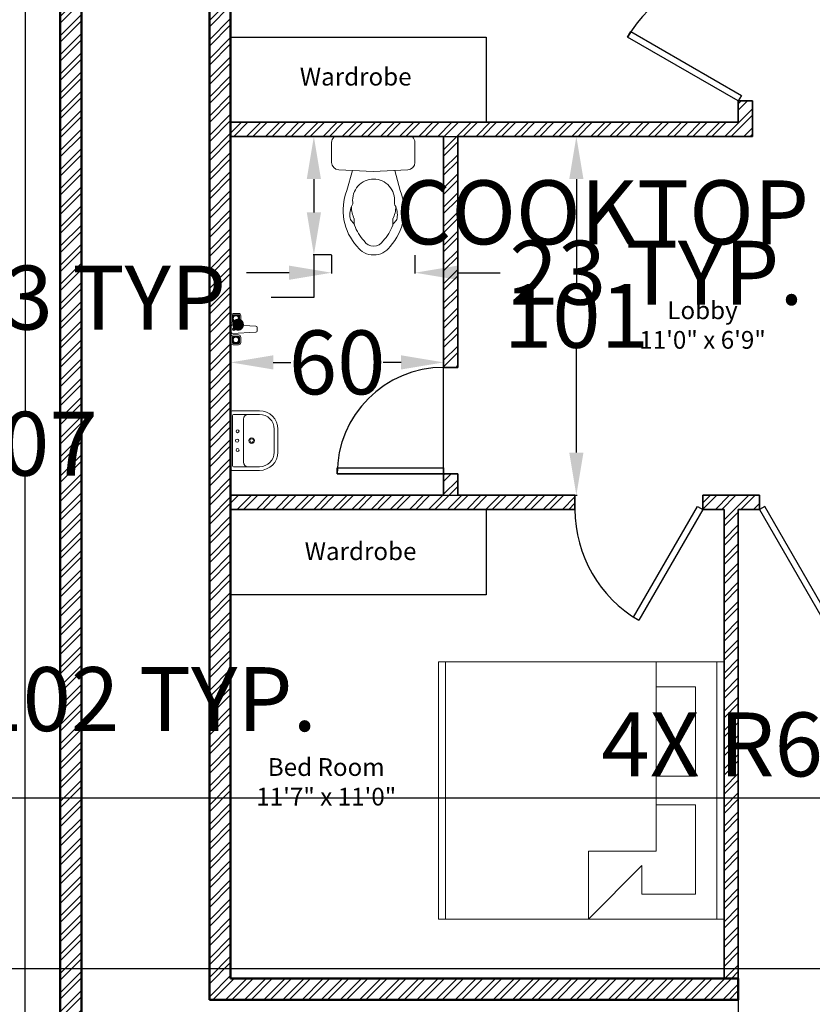
# Model space of a CAD drawing. Units: inches. Extents: x 73 to 1216, y -495 to 328.
# Tile 5 of 9: x 569 to 792, y -232 to 45. Entities that reach past the tile are written whole.
import ezdxf

# ---------------------------------------------------------------- set-up
doc = ezdxf.new("R2010")
doc.units = ezdxf.units.IN
for name, color, linetype, lineweight in [('A-ANNO-DIMS', 2, 'Continuous', 18), ('A-AREA-IDEN', 7, 'Continuous', 18), ('A-DOOR', 3, 'Continuous', 25), ('A-FLOR-CASE', 2, 'Continuous', 25), ('A-FLOR-EDGE', 7, 'Continuous', 25), ('A-FLOR-FIXT', 9, 'Continuous', 18), ('A-WALL-PATT', 8, 'Continuous', 13), ('Furniture', 2, 'Continuous', 18), ('Inner Walls', 5, 'Continuous', 35), ('Outer Walls', 1, 'Continuous', 50), ('Text-T18', 7, 'Continuous', 18)]:
    doc.layers.add(name, color=color, linetype=linetype, lineweight=lineweight)
doc.styles.get("Standard").update_dxf_attribs({"font": 'arial.ttf'})
doc.dimstyles.get("Standard").update_dxf_attribs({"dimtxt": 18, "dimasz": 12, "dimexe": 0.18, "dimexo": 0.0625, "dimgap": 0.09, "dimtad": 0, "dimtih": 1, "dimtoh": 1, "dimdec": 0, "dimzin": 0, "dimdsep": 46, "dimlunit": 3, "dimtxsty": 'Standard', "dimcen": 0.09, "dimadec": 0, "dimazin": 0, "dimtfac": 1, "dimtdec": 0, "dimtofl": 0, "dimtmove": 0, "dimatfit": 3, "dimfxl": 1, "dimtolj": 1, "dimtzin": 0, "dimarcsym": 0})
pattern_1 = [(45, (-647.324, -1257.0093), (-2.694077, 2.694077), []), (45, (-645.528, -1257.0093), (-2.694077, 2.694077), [])]

# ---------------------------------------------------------------- blocks, each defined once
blk = doc.blocks.new('*U2')
for p, q in [((0, 0), (0, -4)), ((36, 0), (36, -4))]:
    blk.add_line(p, q)
blk.add_lwpolyline([(0, 0), (18, 31.18), (19.52, 30.3), (1.52, -0.88)], close=True)
blk.add_arc((0, 0), 36, 0, 60)
blk = doc.blocks.new('*U22')
for p, q in [((0, 0), (0, -4)), ((30, 0), (30, -4))]:
    blk.add_line(p, q)
blk.add_lwpolyline([(0, 0), (0, 30), (1.75, 30), (1.75, 0)], close=True)
blk.add_arc((0, 0), 30, 0, 90)
blk = doc.blocks.new('*U4')
for p, q in [((0, 0), (0, -4)), ((40, 0), (40, -4))]:
    blk.add_line(p, q)
blk.add_lwpolyline([(0, 0), (20, 34.64), (21.52, 33.77), (1.52, -0.88)], close=True)
blk.add_arc((0, 0), 40, 0, 60)
blk = doc.blocks.new('A$C1308471B')
at = {"ltscale": 20}
for p, q in [((0, 0.4607), (0, 0.0186)), ((0.0354, 0.4793), (0.1495, 0.4793)), ((0.2013, 0.2397), (0.1923, 0.4384)), ((0.1957, 0.3639), (0.3109, 0.3953)), ((0.5021, 0.3528), (0.4724, 0.3528)), ((0.4982, 0.3575), (0.4822, 0.3709)), ((0.2013, 0.2397), (0.1923, 0.0409)), ((0.1959, 0.1193), (0.3109, 0.0879)), ((0.5021, 0.1304), (0.4724, 0.1304)), ((0.4982, 0.1257), (0.4822, 0.1123)), ((0.0354, 0), (0.1495, 0))]:
    blk.add_line(p, q, dxfattribs=at)
for centre, radius, start, end in [((0.006, 0.4607), 0.006, 136.5269, 180), ((0.0354, 0.4328), 0.0465, 90, 136.5269), ((0.1495, 0.4365), 0.0429, 2.5755, 90), ((0.4248, 0.1104), 0.3068, 47.4135, 111.7924), ((0.3654, 0.2416), 0.1206, 83.3523, 180), ((0.3823, 0.3868), 0.0255, 263.3523, 298.5742), ((0.4494, 0.2636), 0.1148, 79.3968, 118.5742), ((0.405, 0.2159), 0.153, 63.502, 90.4522), ((0.4658, 0.3513), 0.0255, 50, 79.3968), ((0.5146, 0.377), 0.0255, 230, 251.3881), ((0.5021, 0.3273), 0.0255, 70.3751, 90), ((0.4248, 0.1104), 0.2558, 46.612, 70.3751), ((0.5654, 0.2416), 0.065, 0, 57.2974), ((0.5654, 0.2416), 0.116, 0, 54.7115), ((0.3654, 0.2416), 0.1206, 180, 276.6477), ((0.5654, 0.2416), 0.065, 302.7026, 0), ((0.5654, 0.2416), 0.116, 305.2885, 0), ((0.4248, 0.3728), 0.2558, 289.6249, 313.388), ((0.4248, 0.3728), 0.3068, 248.2076, 312.5865), ((0.3823, 0.0964), 0.0255, 61.4258, 96.6477), ((0.4494, 0.2196), 0.1148, 241.4258, 280.6032), ((0.405, 0.2673), 0.153, 269.5478, 296.498), ((0.5146, 0.1062), 0.0255, 108.6119, 130), ((0.5021, 0.1559), 0.0255, 270, 289.6249), ((0.4658, 0.1319), 0.0255, 280.6032, 310), ((0.006, 0.0186), 0.006, 180, 223.4731), ((0.0354, 0.0465), 0.0465, 223.4731, 270), ((0.1495, 0.0429), 0.0429, 270, 357.4245)]:
    blk.add_arc(centre, radius, start, end, dxfattribs=at)
blk = doc.blocks.new('A$C57EA129C')
for p, q in [((0, 0.4428), (0, 0.1782)), ((0.016, 0.4589), (0.5631, 0.4589)), ((0.0356, 0.4321), (0.0356, 0.2896)), ((0.0445, 0.441), (0.5346, 0.441)), ((0.5435, 0.4321), (0.5435, 0.2896)), ((0.5791, 0.4428), (0.5791, 0.1782)), ((0.0356, 0.2896), (0.0356, 0.1782)), ((0.0802, 0.3341), (0.499, 0.3341)), ((0.5435, 0.2896), (0.5435, 0.1782)), ((0.1782, 0.0356), (0.4009, 0.0356)), ((0.1782, 0), (0.4009, 0))]:
    blk.add_line(p, q)
for centre, radius in [((0.1982, 0.392), 0.0143), ((0.2896, 0.3965), 0.0156), ((0.3809, 0.392), 0.0143), ((0.2896, 0.2545), 0.0267), ((0.2896, 0.2545), 0.0178)]:
    blk.add_circle(centre, radius)
for centre, radius, start, end in [((0.016, 0.4428), 0.016, 90, 180), ((0.0445, 0.4321), 0.00891, 90, 180), ((0.5346, 0.4321), 0.00891, 0, 90), ((0.5631, 0.4428), 0.016, 0, 90), ((0.0802, 0.2896), 0.0445, 90, 180), ((0.499, 0.2896), 0.0445, 0, 90), ((0.1782, 0.1782), 0.1782, 180, 270), ((0.1782, 0.1782), 0.1426, 180, 270), ((0.4009, 0.1782), 0.1782, 270, 0), ((0.4009, 0.1782), 0.1426, 270, 0)]:
    blk.add_arc(centre, radius, start, end)
blk = doc.blocks.new('A$C68D75330')
for p, q in [((0.1549, 0.4064), (0.1549, 0.4514)), ((0.1674, 0.4039), (0.1674, 0.4539)), ((0.1724, 0.4589), (0.2224, 0.4589)), ((0.1749, 0.4714), (0.2199, 0.4714)), ((0.2274, 0.4539), (0.2274, 0.4039)), ((0.2399, 0.4514), (0.2399, 0.4064)), ((0.2644, 0.2559), (0.2524, 0.4614)), ((0.2749, 0.4714), (0.3049, 0.4714)), ((0.3274, 0.4614), (0.3155, 0.2559)), ((0.3399, 0.4514), (0.3399, 0.4064)), ((0.3524, 0.4539), (0.3524, 0.4039)), ((0.4074, 0.4589), (0.3574, 0.4589)), ((0.4049, 0.4714), (0.3599, 0.4714)), ((0.4124, 0.4039), (0.4124, 0.4539)), ((0.4249, 0.4064), (0.4249, 0.4514)), ((0.2224, 0.3989), (0.1724, 0.3989)), ((0.2199, 0.3864), (0.1749, 0.3864)), ((0.3574, 0.3989), (0.4074, 0.3989)), ((0.3599, 0.3864), (0.4049, 0.3864)), ((0.3055, 0.2464), (0.2744, 0.2464))]:
    blk.add_line(p, q)
for centre, radius in [((0.1974, 0.4289), 0.03), ((0.1974, 0.4289), 0.0232), ((0.2899, 0.4464), 0.0125), ((0.2899, 0.4464), 0.00625), ((0.3824, 0.4289), 0.03), ((0.3824, 0.4289), 0.0232)]:
    blk.add_circle(centre, radius)
for centre, radius, start, end in [((0.1749, 0.4514), 0.02, 90, 180), ((0.1724, 0.4539), 0.005, 90, 180), ((0.2199, 0.4514), 0.02, 0, 90), ((0.2224, 0.4539), 0.005, 0, 90), ((0.2736, 0.4441), 0.0273, 87.19754, 140.72744), ((0.3063, 0.4441), 0.0273, 39.27256, 92.80246), ((0.3599, 0.4514), 0.02, 90, 180), ((0.3574, 0.4539), 0.005, 90, 180), ((0.4049, 0.4514), 0.02, 0, 90), ((0.4074, 0.4539), 0.005, 0, 90), ((0.1749, 0.4064), 0.02, 180, 270), ((0.1724, 0.4039), 0.005, 180, 270), ((0.2199, 0.4064), 0.02, 270, 0), ((0.2224, 0.4039), 0.005, 270, 0), ((0.3599, 0.4064), 0.02, 180, 270), ((0.3574, 0.4039), 0.005, 180, 270), ((0.4049, 0.4064), 0.02, 270, 0), ((0.4074, 0.4039), 0.005, 270, 0), ((0.2744, 0.2564), 0.01, 183.3274, 270), ((0.3055, 0.2564), 0.01, 270, 356.6726)]:
    blk.add_arc(centre, radius, start, end)
blk = doc.blocks.new('KING-00')
for p, q in [((-0.8967, -0.947), (-0.8967, 0.8818)), ((0.6019, 0.8818), (0.6019, -0.4644)), ((1.0337, -0.947), (1.0337, 0.8818)), ((0.6019, 0.704), (0.8813, 0.704)), ((0.8813, 0.069), (0.8813, 0.704)), ((0.6019, 0.069), (0.8813, 0.069)), ((0.8813, -0.1342), (0.6019, -0.1342)), ((0.8813, -0.7692), (0.8813, -0.1342)), ((0.1193, -0.4644), (0.1193, -0.947)), ((0.6019, -0.4644), (0.1193, -0.4644)), ((0.1193, -0.947), (0.5003, -0.566)), ((0.5003, -0.7692), (0.5003, -0.566)), ((0.5003, -0.7692), (0.8813, -0.7692))]:
    blk.add_line(p, q)
blk.add_lwpolyline([(-0.9475, -0.947), (-0.9475, 0.8818), (1.0845, 0.8818), (1.0845, -0.947)], close=True)
blk = doc.blocks.new('WARDROBE-72X24')
blk.add_lwpolyline([(0, 24), (72, 24), (72, 0), (0, 0)], close=True)
blk = doc.blocks.new('*D26')
at = {"layer": 'A-ANNO-DIMS', "color": 0, "lineweight": -2, "transparency": 16777216}
for p, q in [((690.69, 91.4), (690.69, 79.21)), ((771.16, 91.4), (771.16, 79.21)), ((702.69, 79.39), (759.16, 79.39)), ((771.16, 79.39), (783.16, 79.39))]:
    blk.add_line(p, q, dxfattribs=at)
at = {"layer": 'A-ANNO-DIMS', "color": 0, "transparency": 16777216}
for points in [[(702.69, 81.39), (702.69, 77.39), (690.69, 79.39)], [(759.16, 81.39), (759.16, 77.39), (771.16, 79.39)]]:
    blk.add_solid(points, dxfattribs=at)
at = {"layer": 'Defpoints', "color": 0, "transparency": 16777216}
for p in [(690.69, 91.46), (771.16, 91.46), (771.16, 79.39)]:
    blk.add_point(p, dxfattribs=at)
at = {"layer": 'A-ANNO-DIMS', "color": 0, "transparency": 16777216, "insert": (890.24, 79.39), "char_height": 18, "attachment_point": 5}
blk.add_mtext('\\A1;KING BED 80 TYP.', dxfattribs=at)
blk = doc.blocks.new('*D28')
at = {"layer": 'A-ANNO-DIMS', "color": 0, "lineweight": -2, "transparency": 16777216}
for p, q in [((520.8, -95.45), (536.15, -95.45)), ((535.97, -107.45), (535.97, -136.81)), ((535.97, -184.97), (535.97, -155.61)), ((520.8, -196.97), (536.15, -196.97))]:
    blk.add_line(p, q, dxfattribs=at)
at = {"layer": 'A-ANNO-DIMS', "color": 0, "transparency": 16777216}
for points in [[(533.97, -107.45), (537.97, -107.45), (535.97, -95.45)], [(533.97, -184.97), (537.97, -184.97), (535.97, -196.97)]]:
    blk.add_solid(points, dxfattribs=at)
at = {"layer": 'Defpoints', "color": 0, "transparency": 16777216}
for p in [(520.74, -95.45), (520.74, -196.97), (535.97, -196.97)]:
    blk.add_point(p, dxfattribs=at)
at = {"layer": 'A-ANNO-DIMS', "color": 0, "transparency": 16777216, "insert": (535.97, -146.21), "char_height": 18, "attachment_point": 5}
blk.add_mtext('\\A1;SECTIONAL 102 TYP.', dxfattribs=at)
blk = doc.blocks.new('*D30')
at = {"layer": 'A-ANNO-DIMS', "color": 0, "lineweight": -2, "transparency": 16777216}
for p, q in [((656.55, 12.18), (651.43, 12.18)), ((651.61, 0.18), (651.61, -9.18)), ((656.55, -21.18), (651.43, -21.18)), ((651.61, -21.18), (651.61, -33.18)), ((651.61, -33.18), (639.61, -33.18))]:
    blk.add_line(p, q, dxfattribs=at)
at = {"layer": 'A-ANNO-DIMS', "color": 0, "transparency": 16777216}
for points in [[(649.61, 0.18), (653.61, 0.18), (651.61, 12.18)], [(649.61, -9.18), (653.61, -9.18), (651.61, -21.18)]]:
    blk.add_solid(points, dxfattribs=at)
at = {"layer": 'Defpoints', "color": 0, "transparency": 16777216}
for p in [(656.61, 12.18), (651.61, -21.18), (656.61, -21.18)]:
    blk.add_point(p, dxfattribs=at)
at = {"layer": 'A-ANNO-DIMS', "color": 0, "transparency": 16777216, "insert": (570.9, -33.18), "char_height": 18, "attachment_point": 5}
blk.add_mtext('\\A1;WC 33 TYP.', dxfattribs=at)
blk = doc.blocks.new('*D31')
at = {"layer": 'A-ANNO-DIMS', "color": 0, "lineweight": -2, "transparency": 16777216}
for p, q in [((656.61, -21.24), (656.61, -26.36)), ((680.08, -21.24), (680.08, -26.36)), ((644.61, -26.18), (632.61, -26.18)), ((692.08, -26.18), (704.08, -26.18))]:
    blk.add_line(p, q, dxfattribs=at)
at = {"layer": 'A-ANNO-DIMS', "color": 0, "transparency": 16777216}
for points in [[(644.61, -24.18), (644.61, -28.18), (656.61, -26.18)], [(692.08, -24.18), (692.08, -28.18), (680.08, -26.18)]]:
    blk.add_solid(points, dxfattribs=at)
at = {"layer": 'Defpoints', "color": 0, "transparency": 16777216}
for p in [(656.61, -21.18), (680.08, -21.18), (680.08, -26.18)]:
    blk.add_point(p, dxfattribs=at)
at = {"layer": 'A-ANNO-DIMS', "color": 0, "transparency": 16777216, "insert": (748.13, -26.18), "char_height": 18, "attachment_point": 5}
blk.add_mtext('\\A1;23 TYP.', dxfattribs=at)
blk = doc.blocks.new('*D42')
at = {"layer": 'A-ANNO-DIMS', "color": 0, "lineweight": -2, "transparency": 16777216}
for p, q in [((903.29, 30.3), (899.05, 30.3)), ((899.23, 18.3), (899.23, 14.82)), ((903.29, 2.82), (899.05, 2.82)), ((899.23, 2.82), (899.23, -9.18)), ((899.23, -9.18), (887.23, -9.18))]:
    blk.add_line(p, q, dxfattribs=at)
at = {"layer": 'A-ANNO-DIMS', "color": 0, "transparency": 16777216}
for points in [[(897.23, 18.3), (901.23, 18.3), (899.23, 30.3)], [(897.23, 14.82), (901.23, 14.82), (899.23, 2.82)]]:
    blk.add_solid(points, dxfattribs=at)
at = {"layer": 'Defpoints', "color": 0, "transparency": 16777216}
for p in [(903.36, 30.3), (899.23, 2.82), (903.36, 2.82)]:
    blk.add_point(p, dxfattribs=at)
at = {"layer": 'A-ANNO-DIMS', "color": 0, "transparency": 16777216, "insert": (777.07, -9.18), "char_height": 18, "attachment_point": 5}
blk.add_mtext('\\A1;COOKTOP 27 TYP.', dxfattribs=at)
blk = doc.blocks.new('*D51')
at = {"layer": 'A-ANNO-DIMS', "color": 0, "lineweight": -2, "transparency": 16777216}
for p, q in [((532.94, 279.18), (570.45, 279.18)), ((570.27, 267.18), (570.27, -65.04)), ((570.27, -415.82), (570.27, -83.6)), ((532.94, -427.82), (570.45, -427.82))]:
    blk.add_line(p, q, dxfattribs=at)
at = {"layer": 'A-ANNO-DIMS', "color": 0, "transparency": 16777216}
for points in [[(568.27, 267.18), (572.27, 267.18), (570.27, 279.18)], [(568.27, -415.82), (572.27, -415.82), (570.27, -427.82)]]:
    blk.add_solid(points, dxfattribs=at)
at = {"layer": 'Defpoints', "color": 0, "transparency": 16777216}
for p in [(532.87, 279.18), (570.27, 279.18), (532.87, -427.82)]:
    blk.add_point(p, dxfattribs=at)
at = {"layer": 'A-ANNO-DIMS', "color": 0, "transparency": 16777216, "insert": (570.27, -74.32), "char_height": 18, "attachment_point": 5}
blk.add_mtext('\\A1;707', dxfattribs=at)
blk = doc.blocks.new('*D53')
at = {"layer": 'A-ANNO-DIMS', "color": 0, "lineweight": -2, "transparency": 16777216}
for p, q in [((580.1, 279.18), (542.58, 279.18)), ((542.76, 267.18), (542.76, -65.04)), ((542.76, -415.82), (542.76, -83.6)), ((580.1, -427.82), (542.58, -427.82))]:
    blk.add_line(p, q, dxfattribs=at)
at = {"layer": 'A-ANNO-DIMS', "color": 0, "transparency": 16777216}
for points in [[(540.76, 267.18), (544.76, 267.18), (542.76, 279.18)], [(540.76, -415.82), (544.76, -415.82), (542.76, -427.82)]]:
    blk.add_solid(points, dxfattribs=at)
at = {"layer": 'Defpoints', "color": 0, "transparency": 16777216}
for p in [(542.76, 279.18), (580.16, 279.18), (580.16, -427.82)]:
    blk.add_point(p, dxfattribs=at)
at = {"layer": 'A-ANNO-DIMS', "color": 0, "transparency": 16777216, "insert": (542.76, -74.32), "char_height": 18, "attachment_point": 5}
blk.add_mtext('\\A1;707', dxfattribs=at)
blk = doc.blocks.new('*D59')
at = {"layer": 'A-ANNO-DIMS', "color": 0, "lineweight": -2, "transparency": 16777216}
for p, q in [((628.16, -88.76), (628.16, -51.24)), ((640.16, -51.42), (645.16, -51.42)), ((676.16, -51.42), (671.17, -51.42)), ((688.16, -88.76), (688.16, -51.24))]:
    blk.add_line(p, q, dxfattribs=at)
at = {"layer": 'A-ANNO-DIMS', "color": 0, "transparency": 16777216}
for points in [[(640.16, -49.42), (640.16, -53.42), (628.16, -51.42)], [(676.16, -49.42), (676.16, -53.42), (688.16, -51.42)]]:
    blk.add_solid(points, dxfattribs=at)
at = {"layer": 'Defpoints', "color": 0, "transparency": 16777216}
for p in [(688.16, -51.42), (628.16, -88.82), (688.16, -88.82)]:
    blk.add_point(p, dxfattribs=at)
at = {"layer": 'A-ANNO-DIMS', "color": 0, "transparency": 16777216, "insert": (658.16, -51.42), "char_height": 18, "attachment_point": 5}
blk.add_mtext('\\A1;60', dxfattribs=at)
blk = doc.blocks.new('*D60')
at = {"layer": 'A-ANNO-DIMS', "color": 0, "lineweight": -2, "transparency": 16777216}
for p, q in [((688.23, 12.18), (725.74, 12.18)), ((725.56, 0.18), (725.56, -29.04)), ((725.56, -76.82), (725.56, -47.6)), ((688.23, -88.82), (725.74, -88.82))]:
    blk.add_line(p, q, dxfattribs=at)
at = {"layer": 'A-ANNO-DIMS', "color": 0, "transparency": 16777216}
for points in [[(723.56, 0.18), (727.56, 0.18), (725.56, 12.18)], [(723.56, -76.82), (727.56, -76.82), (725.56, -88.82)]]:
    blk.add_solid(points, dxfattribs=at)
at = {"layer": 'Defpoints', "color": 0, "transparency": 16777216}
for p in [(688.16, 12.18), (688.16, -88.82), (725.56, -88.82)]:
    blk.add_point(p, dxfattribs=at)
at = {"layer": 'A-ANNO-DIMS', "color": 0, "transparency": 16777216, "insert": (725.56, -38.32), "char_height": 18, "attachment_point": 5}
blk.add_mtext('\\A1;101', dxfattribs=at)
blk = doc.blocks.new('*D67')
at = {"layer": 'A-ANNO-DIMS', "color": 0, "lineweight": -2, "transparency": 16777216}
for p, q in [((798.02113, 227.113801), (798.02113, -465.403699)), ((834.02113, 227.113801), (834.02113, -465.403699)), ((786.02113, -465.223699), (774.02113, -465.223699)), ((846.02113, -465.223699), (858.02113, -465.223699))]:
    blk.add_line(p, q, dxfattribs=at)
at = {"layer": 'A-ANNO-DIMS', "color": 0, "transparency": 16777216}
for points in [[(786.02113, -463.223699), (786.02113, -467.223699), (798.02113, -465.223699)], [(846.02113, -463.223699), (846.02113, -467.223699), (834.02113, -465.223699)]]:
    blk.add_solid(points, dxfattribs=at)
at = {"layer": 'Defpoints', "color": 0, "transparency": 16777216}
for p in [(798.02113, 227.176301), (834.02113, 227.176301), (834.02113, -465.223699)]:
    blk.add_point(p, dxfattribs=at)
at = {"layer": 'A-ANNO-DIMS', "color": 0, "transparency": 16777216, "insert": (816.02113, -465.223699), "char_height": 18, "attachment_point": 5}
blk.add_mtext('\\A1;36', dxfattribs=at)
blk = doc.blocks.new('*D78')
at = {"layer": 'A-ANNO-DIMS', "color": 0, "lineweight": -2, "transparency": 16777216}
for p, q in [((831.3, -174.14), (542.58, -174.14)), ((542.76, -186.14), (542.76, -188.86)), ((542.76, -210.14), (542.76, -207.42)), ((831.3, -222.14), (542.58, -222.14))]:
    blk.add_line(p, q, dxfattribs=at)
at = {"layer": 'A-ANNO-DIMS', "color": 0, "transparency": 16777216}
for points in [[(540.76, -186.14), (544.76, -186.14), (542.76, -174.14)], [(540.76, -210.14), (544.76, -210.14), (542.76, -222.14)]]:
    blk.add_solid(points, dxfattribs=at)
at = {"layer": 'Defpoints', "color": 0, "transparency": 16777216}
for p in [(542.76, -174.14), (831.36, -174.14), (831.36, -222.14)]:
    blk.add_point(p, dxfattribs=at)
at = {"layer": 'A-ANNO-DIMS', "color": 0, "transparency": 16777216, "insert": (542.76, -198.14), "char_height": 18, "attachment_point": 5}
blk.add_mtext('\\A1;48', dxfattribs=at)
blk = doc.blocks.new('*D79')
at = {"layer": 'A-ANNO-DIMS', "color": 0, "lineweight": -2, "transparency": 16777216}
for p, q in [((798.1, -158.97), (810.1, -158.97)), ((810.1, -158.97), (818.61, -167.44)), ((831.27, -180.14), (831.45, -180.14)), ((831.36, -180.23), (831.36, -180.05))]:
    blk.add_line(p, q, dxfattribs=at)
at = {"layer": 'A-ANNO-DIMS', "color": 0, "transparency": 16777216}
blk.add_solid([(820.02, -166.02), (817.19, -168.86), (827.11, -175.91)], dxfattribs=at)
at = {"layer": 'Defpoints', "color": 0, "transparency": 16777216}
for p in [(827.11, -175.91), (831.36, -180.14)]:
    blk.add_point(p, dxfattribs=at)
at = {"layer": 'A-ANNO-DIMS', "color": 0, "transparency": 16777216, "insert": (763.81, -158.97), "char_height": 18, "attachment_point": 5}
blk.add_mtext('\\A1;4X R6', dxfattribs=at)

msp = doc.modelspace()

# ---------------------------------------------------------------- hatches: boundary and pattern name
at = {"layer": 'A-WALL-PATT'}
h = msp.add_hatch(dxfattribs=at)
h.set_pattern_fill('ANSI32', color=256, scale=0.4)
h.set_pattern_definition(pattern_1)
h.paths.add_polyline_path([(586.1647, 273.1763), (924.1647, 273.1763), (924.1647, -421.8237), (753.1647, -421.8237), (753.1647, -427.8237), (930.1647, -427.8237), (930.1647, 279.1763), (580.1647, 279.1763), (580.1647, -427.8237), (633.1647, -427.8237), (633.1647, -421.8237), (586.1647, -421.8237)])
h = msp.add_hatch(dxfattribs=at)
h.set_pattern_fill('ANSI32', color=256, scale=0.4)
h.set_pattern_definition(pattern_1)
h.paths.add_polyline_path([(685.1647, 201.1763), (679.1647, 201.1763), (679.1647, 206.1763), (675.1647, 206.1763), (675.1647, 201.1763), (586.1647, 201.1763), (586.1647, 197.1763), (685.1647, 197.1763)])
h.paths.add_polyline_path([(679.1647, 273.1763), (675.1647, 273.1763), (675.1647, 236.1763), (679.1647, 236.1763)])
h.paths.add_polyline_path([(775.1647, 201.1763), (772.1647, 201.1763), (772.1647, 273.1763), (768.1647, 273.1763), (768.1647, 249.1763), (768.1647, 201.1763), (721.1647, 201.1763), (721.1647, 197.1763), (771.1647, 197.1763), (771.1647, 58.1763), (775.1647, 58.1763)])
h.paths.add_polyline_path([(798.0211, 233.1763), (772.1647, 233.1763), (772.1647, 227.1763), (798.0211, 227.1763)])
h.paths.add_polyline_path([(870.8232, 233.1763), (834.0211, 233.1763), (834.0211, 227.1763), (870.8232, 227.1763)])
h.paths.add_polyline_path([(924.1647, 233.1763), (906.8232, 233.1763), (906.8232, 227.1763), (924.1647, 227.1763)])
h.paths.add_polyline_path([(924.1647, 83.1763), (775.1647, 83.1763), (775.1647, 79.1763), (924.1647, 79.1763)])
h.paths.add_polyline_path([(775.1647, 22.1763), (771.1647, 22.1763), (771.1647, 16.1763), (628.1647, 16.1763), (628.1647, 12.1763), (775.1647, 12.1763)])
h.paths.add_polyline_path([(692.1647, 12.1763), (688.1647, 12.1763), (688.1647, -52.8237), (692.1647, -52.8237)])
h.paths.add_polyline_path([(924.1647, 39.1763), (824.1647, 39.1763), (824.1647, 35.1763), (924.1647, 35.1763)])
h.paths.add_polyline_path([(874.6647, -29.8237), (864.1647, -29.8237), (824.1647, -29.8237), (824.1647, -87.8237), (817.1647, -87.8237), (817.1647, -91.8237), (844.6647, -91.8237), (844.6647, -87.8237), (828.1647, -87.8237), (828.1647, -33.8237), (874.6647, -33.8237)])
h.paths.add_polyline_path([(924.1647, -29.8237), (910.6647, -29.8237), (910.6647, -33.8237), (924.1647, -33.8237)])
h.paths.add_polyline_path([(924.1647, -87.8237), (904.6647, -87.8237), (904.6647, -91.8237), (924.1647, -91.8237)])
h.paths.add_polyline_path([(777.1647, -88.8237), (761.1647, -88.8237), (761.1647, -92.8237), (767.1647, -92.8237), (767.1647, -224.8237), (771.1647, -224.8237), (771.1647, -92.8237), (777.1647, -92.8237)])
h.paths.add_polyline_path([(725.1647, -88.8237), (628.1647, -88.8237), (628.1647, -92.8237), (725.1647, -92.8237)])
h.paths.add_polyline_path([(692.1647, -82.8237), (688.1647, -82.8237), (688.1647, -88.8237), (692.1647, -88.8237)])
h.paths.add_polyline_path([(767.1647, -313.8237), (924.1647, -313.8237), (924.1647, -307.8237), (763.1647, -307.8237), (763.1647, -421.8237), (767.1647, -421.8237)])
h = msp.add_hatch(dxfattribs=at)
h.set_pattern_fill('ANSI32', color=256, scale=0.4)
h.set_pattern_definition(pattern_1)
h.paths.add_polyline_path([(628.1647, 197.1763), (622.1647, 197.1763), (622.1647, -230.8237), (771.1647, -230.8237), (771.1647, -224.8237), (628.1647, -224.8237)])

# ---------------------------------------------------------------- linework, layer by layer
at = {"layer": 'A-FLOR-EDGE'}
msp.add_line((771.1647, -229.8237), (771.1647, -307.8237), dxfattribs=at)
at = {"layer": 'Inner Walls'}
for p, q in [((771.1647, 22.1763), (771.1647, 16.1763)), ((775.1647, 22.1763), (771.1647, 22.1763)), ((775.1647, 22.1763), (775.1647, 12.1763)), ((771.1647, 16.1763), (628.1647, 16.1763)), ((688.1647, 12.1763), (628.1647, 12.1763)), ((688.1647, -52.8237), (688.1647, 12.1763)), ((775.1647, 12.1763), (692.1647, 12.1763)), ((692.1647, -52.8237), (692.1647, 12.1763)), ((692.1647, -52.8237), (688.1647, -52.8237)), ((692.1647, -82.8237), (658.1647, -82.8237)), ((688.1647, -88.8237), (688.1647, -81.0737)), ((692.1647, -88.8237), (692.1647, -82.8237)), ((688.1647, -88.8237), (628.1647, -88.8237)), ((725.1647, -88.8237), (692.1647, -88.8237)), ((725.1647, -92.8237), (725.1647, -88.8237)), ((761.1647, -92.8237), (761.1647, -88.8237)), ((761.1647, -88.8237), (777.1647, -88.8237)), ((777.1647, -88.8237), (777.1647, -92.8237)), ((725.1647, -92.8237), (628.1647, -92.8237)), ((767.1647, -92.8237), (761.1647, -92.8237)), ((767.1647, -224.8237), (767.1647, -92.8237)), ((771.1647, -224.8237), (771.1647, -92.8237)), ((771.1647, -92.8237), (777.1647, -92.8237))]:
    msp.add_line(p, q, dxfattribs=at)
at = {"layer": 'Outer Walls'}
for p, q in [((580.1647, -427.8237), (580.1647, 279.1763)), ((586.1647, -421.8237), (586.1647, 273.1763)), ((622.1647, -230.8237), (622.1647, 197.1763)), ((628.1647, -224.8237), (628.1647, 197.1763)), ((771.1647, -224.8237), (628.1647, -224.8237)), ((771.1647, -224.8237), (771.1647, -230.8237)), ((771.1647, -230.8237), (622.1647, -230.8237))]:
    msp.add_line(p, q, dxfattribs=at)

# ---------------------------------------------------------------- block references
at = {"layer": 'A-DOOR'}
for name, p, rotation in [('*U2', (771.1647, 22.1763), 90), ('*U22', (688.1647, -82.8237), 90.00000000000003), ('*U2', (761.1647, -92.8237), 180)]:
    msp.add_blockref(name, p, dxfattribs=dict(at, rotation=rotation))
at = {"layer": 'A-DOOR', "xscale": -1, "rotation": 180}
msp.add_blockref('*U4', (777.1647, -92.8237), dxfattribs=at)
at = {"layer": 'A-FLOR-CASE'}
for p in [(628.1651, 16.176), (628.1651, -116.824)]:
    msp.add_blockref('WARDROBE-72X24', p, dxfattribs=at)
at = {"layer": 'A-FLOR-FIXT'}
for name, p, xscale, yscale, zscale, rotation in [('A$C1308471B', (656.6088, 12.1763), 48.95497407897215, 48.95497407897215, 48.95497407897215, 269.9999999999999), ('A$C68D75330', (643.6487, -51.536), 32.67217261962217, 32.67217261962217, 32.67217261962217, 89.99999999999999), ('A$C57EA129C', (641.4641, -65.051), -28.98333223671166, 28.98333223671166, 28.98333223671166, 90)]:
    msp.add_blockref(name, p, dxfattribs=dict(at, xscale=xscale, yscale=yscale, zscale=zscale, rotation=rotation))
at = {"layer": 'Furniture', "xscale": 39.60249106241186, "yscale": 39.60249106241186, "zscale": 39.60249106241186}
msp.add_blockref('KING-00', (724.2158, -170.639), dxfattribs=at)

# ---------------------------------------------------------------- texts
at = {"layer": 'A-AREA-IDEN', "char_height": 5, "attachment_point": 3}
for s, insert in [('\\pxqc;{\\fTimes New Roman|b0|i0|c0|p18;Lobby\\P11\'0" x 6\'9"}', (785.6525, -34.2468)), ('\\pxqc;{\\fTimes New Roman|b0|i0|c0|p18;Bed Room \\P11\'7" x 11\'0"}', (679.6433, -162.8344))]:
    msp.add_mtext_dynamic_manual_height_columns(s, width=49.101878, gutter_width=12.5, heights=[0], dxfattribs=dict(at, insert=insert))
at = {"layer": 'Text-T18', "char_height": 5, "attachment_point": 3}
for insert in [(687.9442, 31.5208), (689.3169, -102.0799)]:
    msp.add_mtext_dynamic_manual_height_columns('\\pxqc;{\\fTimes New Roman|b0|i0|c0|p18;Wardrobe}', width=49.101878, gutter_width=12.5, heights=[0], dxfattribs=dict(at, insert=insert))

# ---------------------------------------------------------------- dimensions: what is measured, and where the dimension line sits
at = {"layer": 'A-ANNO-DIMS'}
for base, p1, p2, angle, picture, middle in [((542.7647, 279.1763), (580.1647, -427.8237), (580.1647, 279.1763), 90, '*D53', (542.7647, -74.3237)), ((570.2746, 279.1763), (532.8746, -427.8237), (532.8746, 279.1763), 90, '*D51', (570.2746, -74.3237)), ((725.5647, -88.8237), (688.1647, 12.1763), (688.1647, -88.8237), 270, '*D60', (725.5647, -38.3237)), ((688.1647, -51.4237), (628.1647, -88.8237), (688.1647, -88.8237), 0, '*D59', (658.1647, -51.4237)), ((542.7647, -174.1414), (831.3578, -222.1414), (831.3578, -174.1414), 90, '*D78', (542.7647, -198.1414))]:
    dim = msp.add_linear_dim(base=base, p1=p1, p2=p2, angle=angle, dimstyle='Standard', override={"dimdec": 0, "dimlfac": 1, "dimrnd": 0, "dimzin": 0, "dimdsep": 46, "dimlunit": 2}, dxfattribs=at)
    dim.commit()
    dim.dimension.update_dxf_attribs({"geometry": picture, "text_midpoint": middle})
dim = msp.add_linear_dim(base=(834.0211, -465.2237), p1=(798.0211, 227.1763), p2=(834.0211, 227.1763), dimstyle='Standard', override={"dimdec": 0, "dimlfac": 1, "dimrnd": 0, "dimzin": 0, "dimdsep": 46, "dimlunit": 2}, dxfattribs=at)
dim.commit()
dim.dimension.update_dxf_attribs({"geometry": '*D67', "text_midpoint": (816.0211, -465.2237)})
for base, p1, p2, text, picture, middle in [((771.1647, 79.3929), (690.6924, 91.4638), (771.1647, 91.4638), 'KING BED <> TYP.', '*D26', (890.2417, 79.3929)), ((680.0753, -26.184), (656.6088, -21.1805), (680.0753, -21.1805), '<> TYP.', '*D31', (748.1278, -26.184))]:
    dim = msp.add_linear_dim(base=base, p1=p1, p2=p2, text=text, dimstyle='Standard', override={"dimdec": 0, "dimlfac": 1, "dimrnd": 0, "dimzin": 0, "dimdsep": 46, "dimlunit": 2}, dxfattribs=at)
    dim.commit()
    dim.dimension.update_dxf_attribs({"geometry": picture, "text_midpoint": middle})
for base, p1, p2, text, picture, middle in [((899.2332, 2.82), (903.3556, 30.303), (903.3556, 2.82), 'COOKTOP <> TYP.', '*D42', (777.0743, -9.18)), ((651.6053, -21.1805), (656.6088, 12.1763), (656.6088, -21.1805), 'WC <> TYP.', '*D30', (570.898, -33.1805)), ((535.9692, -196.9696), (520.7411, -95.4493), (520.7411, -196.9696), 'SECTIONAL <> TYP.', '*D28', (535.9692, -146.2095))]:
    dim = msp.add_linear_dim(base=base, p1=p1, p2=p2, angle=270, text=text, dimstyle='Standard', override={"dimdec": 0, "dimlfac": 1, "dimrnd": 0, "dimzin": 0, "dimdsep": 46, "dimlunit": 2}, dxfattribs=at)
    dim.commit()
    dim.dimension.update_dxf_attribs({"geometry": picture, "text_midpoint": middle})
dim = msp.add_radius_dim(center=(831.3578, -180.1414), mpoint=(827.107, -175.9069), text='4X <>', dimstyle='Standard', override={"dimdec": 0, "dimlfac": 1, "dimrnd": 0, "dimzin": 0, "dimdsep": 46, "dimlunit": 2}, dxfattribs=at)
dim.commit()
dim.dimension.update_dxf_attribs({"geometry": '*D79', "text_midpoint": (763.8062, -158.9692)})

doc.saveas('drawing.dxf')
